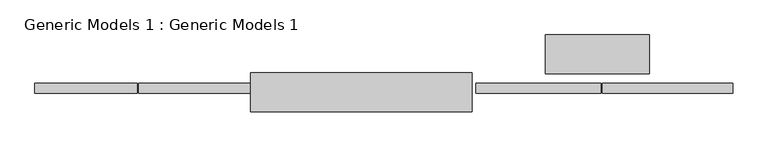
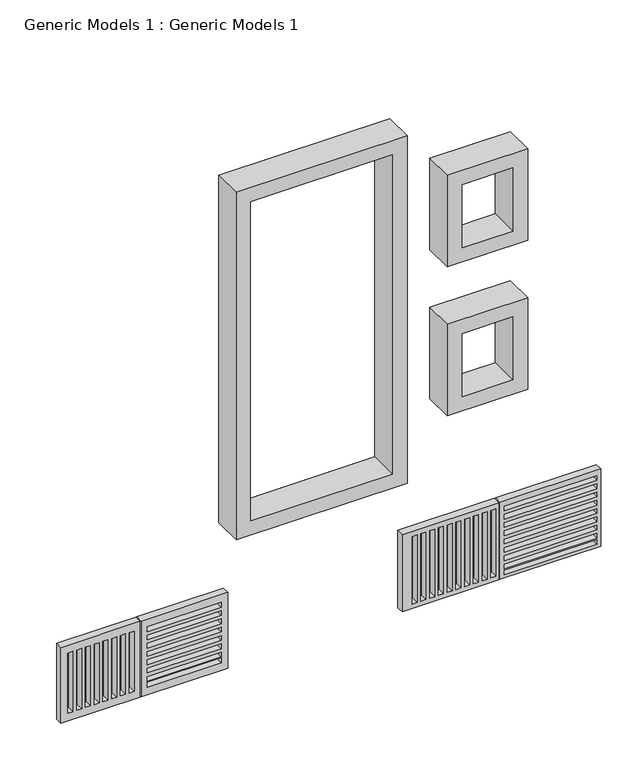
"""IFC4 building model written with IfcOpenShell, lengths in millimetres: proxy geometry, Generic Models 1 : Generic Models 1."""

from ifc_helpers import new_model, si_unit, frame, origin, place, context, project, spatial, polyline, outline, extrude, source, transform, mapped, element, save


def generic_models_1_generic_models_1_6b654720(model_context):
    return source(origin(), model_context, "Body", "SweptSolid", [
        extrude(outline(polyline([(85.2892439, 4204.3134019), (1745.6727273, 4204.3134019), (1745.6727273, 2154.8530765), (85.2892439, 2154.8530765), (85.2892439, 4204.3134019)]), holes=[polyline([(1527.7666374, 2245.8756691), (1629.3666374, 2245.8756691), (1629.3666374, 4125.4756691), (1527.7666374, 4125.4756691), (1527.7666374, 2245.8756691)]), polyline([(1349.9666374, 2245.8756691), (1451.5666374, 2245.8756691), (1451.5666374, 4125.4756691), (1349.9666374, 4125.4756691), (1349.9666374, 2245.8756691)]), polyline([(1172.1666374, 2245.8756691), (1273.7666374, 2245.8756691), (1273.7666374, 4125.4756691), (1172.1666374, 4125.4756691), (1172.1666374, 2245.8756691)]), polyline([(994.3666374, 2245.8756691), (1095.9666374, 2245.8756691), (1095.9666374, 4125.4756691), (994.3666374, 4125.4756691), (994.3666374, 2245.8756691)]), polyline([(816.5666374, 2245.8756691), (918.1666374, 2245.8756691), (918.1666374, 4125.4756691), (816.5666374, 4125.4756691), (816.5666374, 2245.8756691)]), polyline([(638.7666374, 2245.8756691), (740.3666374, 2245.8756691), (740.3666374, 4125.4756691), (638.7666374, 4125.4756691), (638.7666374, 2245.8756691)]), polyline([(460.9666374, 2245.8756691), (562.5666374, 2245.8756691), (562.5666374, 4125.4756691), (460.9666374, 4125.4756691), (460.9666374, 2245.8756691)]), polyline([(283.1666374, 2245.8756691), (384.7666374, 2245.8756691), (384.7666374, 4125.4756691), (283.1666374, 4125.4756691), (283.1666374, 2245.8756691)]), polyline([(149.8166374, 2245.8756691), (251.4166374, 2245.8756691), (251.4166374, 4125.4756691), (149.8166374, 4125.4756691), (149.8166374, 2245.8756691)])]), frame((0.0, -8733.8212413, 0.0), z_axis=(0.0, 1.0, 0.0), x_axis=(0.0, 0.0, 1.0)), (0.0, 0.0, 1.0), 152.4),
        extrude(outline(polyline([(1745.6727273, 165.7134019), (85.2892439, 165.7134019), (85.2892439, 2130.4671371), (1745.6727273, 2130.4671371), (1745.6727273, 165.7134019)]), holes=[polyline([(181.5666374, 373.0804549), (1629.3666374, 373.0804549), (1629.3666374, 474.6804549), (181.5666374, 474.6804549), (181.5666374, 373.0804549)]), polyline([(181.5666374, 550.8804549), (1629.3666374, 550.8804549), (1629.3666374, 652.4804549), (181.5666374, 652.4804549), (181.5666374, 550.8804549)]), polyline([(181.5666374, 728.6804549), (1629.3666374, 728.6804549), (1629.3666374, 830.2804549), (181.5666374, 830.2804549), (181.5666374, 728.6804549)]), polyline([(181.5666374, 906.4804549), (1629.3666374, 906.4804549), (1629.3666374, 1008.0804549), (181.5666374, 1008.0804549), (181.5666374, 906.4804549)]), polyline([(181.5666374, 1084.2804549), (1629.3666374, 1084.2804549), (1629.3666374, 1185.8804549), (181.5666374, 1185.8804549), (181.5666374, 1084.2804549)]), polyline([(181.5666374, 1262.0804549), (1629.3666374, 1262.0804549), (1629.3666374, 1363.6804549), (181.5666374, 1363.6804549), (181.5666374, 1262.0804549)]), polyline([(181.5666374, 1439.8804549), (1629.3666374, 1439.8804549), (1629.3666374, 1541.4804549), (181.5666374, 1541.4804549), (181.5666374, 1439.8804549)]), polyline([(181.5666374, 1617.6804549), (1629.3666374, 1617.6804549), (1629.3666374, 1719.2804549), (181.5666374, 1719.2804549), (181.5666374, 1617.6804549)]), polyline([(181.5666374, 1795.4804549), (1629.3666374, 1795.4804549), (1629.3666374, 1897.0804549), (181.5666374, 1897.0804549), (181.5666374, 1795.4804549)]), polyline([(181.5666374, 1973.2804549), (1629.3666374, 1973.2804549), (1629.3666374, 2074.8804549), (181.5666374, 2074.8804549), (181.5666374, 1973.2804549)])]), frame((0.0, -8733.8212413, 0.0), z_axis=(0.0, 1.0, 0.0), x_axis=(0.0, 0.0, 1.0)), (0.0, 0.0, 1.0), 152.4),
        extrude(outline(polyline([(117.5127965, -3377.5865981), (1745.6727273, -3377.5865981), (1745.6727273, -5139.1512458), (117.5127965, -5139.1512458), (117.5127965, -3377.5865981)]), holes=[polyline([(1474.5098516, -5012.0329893), (1576.1098516, -5012.0329893), (1576.1098516, -3513.4329893), (1474.5098516, -3513.4329893), (1474.5098516, -5012.0329893)]), polyline([(1296.7098516, -5012.0329893), (1398.3098516, -5012.0329893), (1398.3098516, -3513.4329893), (1296.7098516, -3513.4329893), (1296.7098516, -5012.0329893)]), polyline([(1118.9098516, -5012.0329893), (1220.5098516, -5012.0329893), (1220.5098516, -3513.4329893), (1118.9098516, -3513.4329893), (1118.9098516, -5012.0329893)]), polyline([(941.1098516, -5012.0329893), (1042.7098516, -5012.0329893), (1042.7098516, -3513.4329893), (941.1098516, -3513.4329893), (941.1098516, -5012.0329893)]), polyline([(763.3098516, -5012.0329893), (864.9098516, -5012.0329893), (864.9098516, -3513.4329893), (763.3098516, -3513.4329893), (763.3098516, -5012.0329893)]), polyline([(585.5098516, -5012.0329893), (687.1098516, -5012.0329893), (687.1098516, -3513.4329893), (585.5098516, -3513.4329893), (585.5098516, -5012.0329893)]), polyline([(407.7098516, -5012.0329893), (509.3098516, -5012.0329893), (509.3098516, -3513.4329893), (407.7098516, -3513.4329893), (407.7098516, -5012.0329893)]), polyline([(280.7098516, -5012.0329893), (382.3098516, -5012.0329893), (382.3098516, -3513.4329893), (280.7098516, -3513.4329893), (280.7098516, -5012.0329893)])]), frame((0.0, -8733.8212413, 0.0), z_axis=(0.0, 1.0, 0.0), x_axis=(0.0, 0.0, 1.0)), (0.0, 0.0, 1.0), 152.4),
        extrude(outline(polyline([(1745.6727273, -6768.4865981), (117.5127965, -6768.4865981), (117.5127965, -5162.6958691), (1745.6727273, -5162.6958691), (1745.6727273, -6768.4865981)]), holes=[polyline([(283.784568, -6625.9610569), (1579.184568, -6625.9610569), (1579.184568, -6524.3610569), (283.784568, -6524.3610569), (283.784568, -6625.9610569)]), polyline([(283.784568, -6448.1610569), (1579.184568, -6448.1610569), (1579.184568, -6346.5610569), (283.784568, -6346.5610569), (283.784568, -6448.1610569)]), polyline([(283.784568, -6270.3610569), (1579.184568, -6270.3610569), (1579.184568, -6168.7610569), (283.784568, -6168.7610569), (283.784568, -6270.3610569)]), polyline([(283.784568, -6092.5610569), (1579.184568, -6092.5610569), (1579.184568, -5990.9610569), (283.784568, -5990.9610569), (283.784568, -6092.5610569)]), polyline([(283.784568, -5914.7610569), (1579.184568, -5914.7610569), (1579.184568, -5813.1610569), (283.784568, -5813.1610569), (283.784568, -5914.7610569)]), polyline([(283.784568, -5736.9610569), (1579.184568, -5736.9610569), (1579.184568, -5635.3610569), (283.784568, -5635.3610569), (283.784568, -5736.9610569)]), polyline([(283.784568, -5559.1610569), (1579.184568, -5559.1610569), (1579.184568, -5457.5610569), (283.784568, -5457.5610569), (283.784568, -5559.1610569)]), polyline([(283.784568, -5381.3610569), (1579.184568, -5381.3610569), (1579.184568, -5279.7610569), (283.784568, -5279.7610569), (283.784568, -5381.3610569)])]), frame((0.0, -8733.8212413, 0.0), z_axis=(0.0, 1.0, 0.0), x_axis=(0.0, 0.0, 1.0)), (0.0, 0.0, 1.0), 152.4),
        extrude(outline(polyline([(8896.35, 2896.2134019), (8896.35, 1257.9134019), (6931.0676291, 1257.9134019), (6931.0676291, 2896.2134019), (8896.35, 2896.2134019)]), holes=[polyline([(8591.55, 2591.4134019), (7235.8676291, 2591.4134019), (7235.8676291, 1562.7134019), (8591.55, 1562.7134019), (8591.55, 2591.4134019)])]), frame((0.0, -8429.0212413, 0.0), z_axis=(0.0, 1.0, 0.0), x_axis=(0.0, 0.0, 1.0)), (0.0, 0.0, 1.0), 609.6),
        extrude(outline(polyline([(5695.95, 2896.2134019), (5695.95, 1257.9134019), (3730.6676291, 1257.9134019), (3730.6676291, 2896.2134019), (5695.95, 2896.2134019)]), holes=[polyline([(5391.15, 2591.4134019), (4035.4676291, 2591.4134019), (4035.4676291, 1562.7134019), (5391.15, 1562.7134019), (5391.15, 2591.4134019)])]), frame((0.0, -8429.0212413, 0.0), z_axis=(0.0, 1.0, 0.0), x_axis=(0.0, 0.0, 1.0)), (0.0, 0.0, 1.0), 609.6),
        extrude(outline(polyline([(10515.6, 102.2134019), (10515.6, -3377.5865981), (3048.0, -3377.5865981), (3048.0, 102.2134019), (10515.6, 102.2134019)]), holes=[polyline([(10210.8, -202.5865981), (3352.8, -202.5865981), (3352.8, -3072.7865981), (10210.8, -3072.7865981), (10210.8, -202.5865981)])]), frame((0.0, -9025.9212413, 0.0), z_axis=(0.0, 1.0, 0.0), x_axis=(0.0, 0.0, 1.0)), (0.0, 0.0, 1.0), 609.6),
    ])


if __name__ == "__main__":
    model = new_model("IFC4")
    model_context = context("Model", 3, world=origin())
    ifc_project = project(units=[si_unit("LENGTHUNIT", "METRE", prefix="MILLI")], contexts=[model_context])
    site = spatial("IfcSite", under=ifc_project)
    building = spatial("IfcBuilding", under=site)
    placement = place(None, origin())
    generic_models_1_generic_models_1_shape = generic_models_1_generic_models_1_6b654720(model_context)
    element("IfcBuildingElementProxy", 1, Name="Generic Models 1 : Generic Models 1", ObjectType="Generic Models 1 : Generic Models 1", at=placement, inside=building, context=model_context, shape_type="MappedRepresentation", body=[
        mapped(generic_models_1_generic_models_1_shape, transform((0.0, 0.0, 0.0), x_axis=(1.0, 0.0, 0.0), y_axis=(0.0, 1.0, 0.0), z_axis=(0.0, 0.0, 1.0))),
    ])
    save(model, "model.ifc")

# Revit data of these elements
# Element 1 (IfcBuildingElementProxy, "Generic Models 1 : Generic Models 1")
#   Materials on its faces: "wood", "Earth"
# Materials
#   "wood": class "Generic", colour RGB 155 131 132, transparency 0, Cost = 0
#   "Earth": class "Generic", colour RGB 97 75 62, transparency 0, Description = "Soil", Cost = 0
